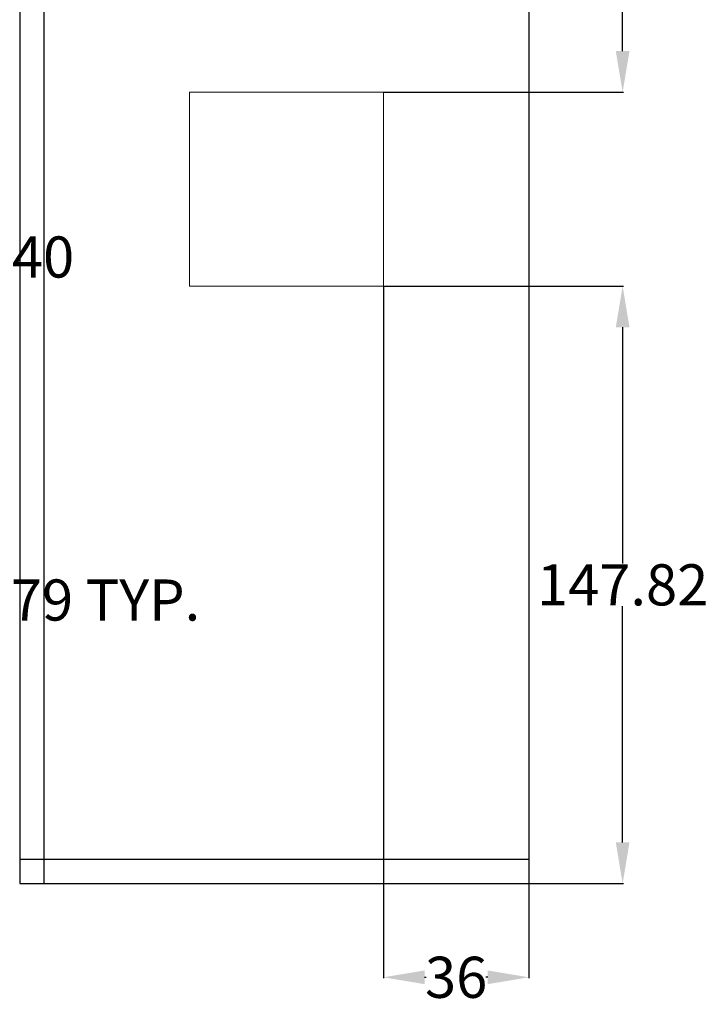
# Model space of a CAD drawing. Units: inches. Extents: x -107 to 647, y -210 to 500.
# Tile 5 of 7: x 477 to 647, y -28 to 216. Entities that reach past the tile are written whole.
import ezdxf

# ---------------------------------------------------------------- set-up
doc = ezdxf.new("R2010")
doc.units = ezdxf.units.IN
doc.header["$MEASUREMENT"] = 0
for name, color, linetype, lineweight in [('A-ANNO-DIMS', 2, 'Continuous', 18), ('A-ELEV', 30, 'Continuous', 25), ('A-ELEV-GLAZ', 4, 'Continuous', 18)]:
    doc.layers.add(name, color=color, linetype=linetype, lineweight=lineweight)
doc.styles.get("Standard").update_dxf_attribs({"font": 'arial.ttf'})
doc.dimstyles.get("Standard").update_dxf_attribs({"dimtxt": 10.18, "dimasz": 10.18, "dimexe": 0.18, "dimexo": 0.0625, "dimgap": 0.09, "dimtad": 0, "dimtih": 1, "dimtoh": 1, "dimdec": 0, "dimzin": 0, "dimdsep": 46, "dimlunit": 3, "dimtxsty": 'Standard', "dimcen": 0.09, "dimadec": 0, "dimazin": 0, "dimtfac": 1, "dimtdec": 0, "dimtofl": 0, "dimtmove": 0, "dimatfit": 3, "dimfxl": 1, "dimtolj": 1, "dimtzin": 0, "dimarcsym": 0})

# ---------------------------------------------------------------- blocks, each defined once
blk = doc.blocks.new('WINDOW-ELEV-48X48IN')
blk.add_lwpolyline([(0, 48), (48, 48), (48, 0), (0, 0)], close=True)
blk = doc.blocks.new('*D48')
at = {"layer": 'A-ANNO-DIMS', "color": 0, "lineweight": -2, "transparency": 16777216}
for p, q in [((288.08, 84.26), (288.08, 72.3)), ((367.08, 84.26), (367.08, 72.3)), ((298.26, 72.48), (356.9, 72.48)), ((367.08, 72.48), (377.26, 72.48))]:
    blk.add_line(p, q, dxfattribs=at)
at = {"layer": 'A-ANNO-DIMS', "color": 0, "transparency": 16777216}
for points in [[(298.26, 74.17), (298.26, 70.78), (288.08, 72.48)], [(356.9, 74.17), (356.9, 70.78), (367.08, 72.48)]]:
    blk.add_solid(points, dxfattribs=at)
at = {"layer": 'Defpoints', "color": 0, "transparency": 16777216}
for p in [(288.08, 84.33), (367.08, 84.33), (367.08, 72.48)]:
    blk.add_point(p, dxfattribs=at)
at = {"layer": 'A-ANNO-DIMS', "color": 0, "transparency": 16777216, "insert": (452.28, 72.48), "char_height": 10.18, "attachment_point": 5}
blk.add_mtext('\\A1;STAIR FLIGHT 79 TYP.', dxfattribs=at)
blk = doc.blocks.new('*D60')
at = {"layer": 'A-ANNO-DIMS', "color": 0, "lineweight": -2, "transparency": 16777216}
for p, q in [((320.6, 163.26), (320.6, 157.18)), ((360.38, 163.26), (360.38, 157.18)), ((330.78, 157.36), (350.2, 157.36)), ((360.38, 157.36), (370.56, 157.36))]:
    blk.add_line(p, q, dxfattribs=at)
at = {"layer": 'A-ANNO-DIMS', "color": 0, "transparency": 16777216}
for points in [[(330.78, 159.06), (330.78, 155.66), (320.6, 157.36)], [(350.2, 159.06), (350.2, 155.66), (360.38, 157.36)]]:
    blk.add_solid(points, dxfattribs=at)
at = {"layer": 'Defpoints', "color": 0, "transparency": 16777216}
for p in [(320.6, 163.33), (360.38, 163.33), (360.38, 157.36)]:
    blk.add_point(p, dxfattribs=at)
at = {"layer": 'A-ANNO-DIMS', "color": 0, "transparency": 16777216, "insert": (433.18, 157.36), "char_height": 10.18, "attachment_point": 5}
blk.add_mtext('\\A1;COFFEE TABLE 40', dxfattribs=at)
blk = doc.blocks.new('*D100')
at = {"layer": 'A-ANNO-DIMS', "color": 0, "lineweight": -2, "transparency": 16777216}
for p, q in [((566.81, 150.15), (626.13, 150.15)), ((625.95, 139.97), (625.95, 81.52)), ((625.95, 12.51), (625.95, 70.95)), ((602.81, 2.33), (626.13, 2.33))]:
    blk.add_line(p, q, dxfattribs=at)
at = {"layer": 'A-ANNO-DIMS', "color": 0, "transparency": 16777216}
for points in [[(624.25, 139.97), (627.65, 139.97), (625.95, 150.15)], [(624.25, 12.51), (627.65, 12.51), (625.95, 2.33)]]:
    blk.add_solid(points, dxfattribs=at)
at = {"layer": 'Defpoints', "color": 0, "transparency": 16777216}
for p in [(566.75, 150.15), (625.95, 150.15), (602.75, 2.33)]:
    blk.add_point(p, dxfattribs=at)
at = {"layer": 'A-ANNO-DIMS', "color": 0, "transparency": 16777216, "insert": (625.95, 76.24), "char_height": 10.18, "attachment_point": 5}
blk.add_mtext('\\A1;147.82', dxfattribs=at)
blk = doc.blocks.new('*D101')
at = {"layer": 'A-ANNO-DIMS', "color": 0, "lineweight": -2, "transparency": 16777216}
for p, q in [((566.81, 399.2), (626.13, 399.2)), ((625.95, 389.02), (625.95, 303.96)), ((625.95, 208.33), (625.95, 293.39)), ((566.81, 198.15), (626.13, 198.15))]:
    blk.add_line(p, q, dxfattribs=at)
at = {"layer": 'A-ANNO-DIMS', "color": 0, "transparency": 16777216}
for points in [[(624.25, 389.02), (627.65, 389.02), (625.95, 399.2)], [(624.25, 208.33), (627.65, 208.33), (625.95, 198.15)]]:
    blk.add_solid(points, dxfattribs=at)
at = {"layer": 'Defpoints', "color": 0, "transparency": 16777216}
for p in [(566.75, 399.2), (625.95, 399.2), (566.75, 198.15)]:
    blk.add_point(p, dxfattribs=at)
at = {"layer": 'A-ANNO-DIMS', "color": 0, "transparency": 16777216, "insert": (625.95, 298.67), "char_height": 10.18, "attachment_point": 5}
blk.add_mtext('\\A1;201.05', dxfattribs=at)
blk = doc.blocks.new('*D102')
at = {"layer": 'A-ANNO-DIMS', "color": 0, "lineweight": -2, "transparency": 16777216}
for p, q in [((566.75, 150.09), (566.75, -21.05)), ((602.75, 2.26), (602.75, -21.05)), ((576.93, -20.87), (577.37, -20.87)), ((592.57, -20.87), (592.12, -20.87))]:
    blk.add_line(p, q, dxfattribs=at)
at = {"layer": 'A-ANNO-DIMS', "color": 0, "transparency": 16777216}
for points in [[(576.93, -19.18), (576.93, -22.57), (566.75, -20.87)], [(592.57, -19.18), (592.57, -22.57), (602.75, -20.87)]]:
    blk.add_solid(points, dxfattribs=at)
at = {"layer": 'Defpoints', "color": 0, "transparency": 16777216}
for p in [(566.75, 150.15), (602.75, 2.33), (602.75, -20.87)]:
    blk.add_point(p, dxfattribs=at)
at = {"layer": 'A-ANNO-DIMS', "color": 0, "transparency": 16777216, "insert": (584.75, -20.87), "char_height": 10.18, "attachment_point": 5}
blk.add_mtext('\\A1;36', dxfattribs=at)

msp = doc.modelspace()

# ---------------------------------------------------------------- linework, layer by layer
at = {"layer": 'A-ELEV'}
for p, q in [((476.749, 464.325), (476.749, 2.325)), ((482.749, 464.325), (482.749, 2.325)), ((602.749, 464.325), (602.749, 2.325)), ((476.749, 8.325), (602.749, 8.325)), ((476.749, 2.325), (602.749, 2.325))]:
    msp.add_line(p, q, dxfattribs=at)

# ---------------------------------------------------------------- block references
at = {"layer": 'A-ELEV-GLAZ'}
msp.add_blockref('WINDOW-ELEV-48X48IN', (518.749, 150.148), dxfattribs=at)

# ---------------------------------------------------------------- dimensions: what is measured, and where the dimension line sits
at = {"layer": 'A-ANNO-DIMS'}
for base, p1, p2, picture, middle in [((625.949, 399.198), (566.749, 198.148), (566.749, 399.198), '*D101', (625.949, 298.673)), ((625.949, 150.148), (602.749, 2.325), (566.749, 150.148), '*D100', (625.949, 76.237))]:
    dim = msp.add_linear_dim(base=base, p1=p1, p2=p2, angle=90, dimstyle='Standard', override={"dimdec": 2, "dimlfac": 1, "dimrnd": 0, "dimzin": 0, "dimdsep": 46, "dimlunit": 2}, dxfattribs=at)
    dim.commit()
    dim.dimension.update_dxf_attribs({"geometry": picture, "text_midpoint": middle})
for base, p1, p2, text, picture, middle in [((360.376, 157.36), (320.599, 163.327), (360.376, 163.327), 'COFFEE TABLE <>', '*D60', (433.177, 157.36)), ((367.082, 72.475), (288.082, 84.325), (367.082, 84.325), 'STAIR FLIGHT <> TYP.', '*D48', (452.278, 72.475))]:
    dim = msp.add_linear_dim(base=base, p1=p1, p2=p2, text=text, dimstyle='Standard', override={"dimdec": 0, "dimlfac": 1, "dimrnd": 0, "dimzin": 0, "dimdsep": 46, "dimlunit": 2}, dxfattribs=at)
    dim.commit()
    dim.dimension.update_dxf_attribs({"geometry": picture, "text_midpoint": middle})
dim = msp.add_linear_dim(base=(602.749, -20.875), p1=(566.749, 150.148), p2=(602.749, 2.325), dimstyle='Standard', override={"dimdec": 0, "dimlfac": 1, "dimrnd": 0, "dimzin": 0, "dimdsep": 46, "dimlunit": 2}, dxfattribs=at)
dim.commit()
dim.dimension.update_dxf_attribs({"geometry": '*D102', "text_midpoint": (584.749, -20.875)})

doc.saveas('drawing.dxf')
